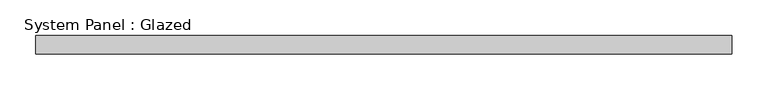
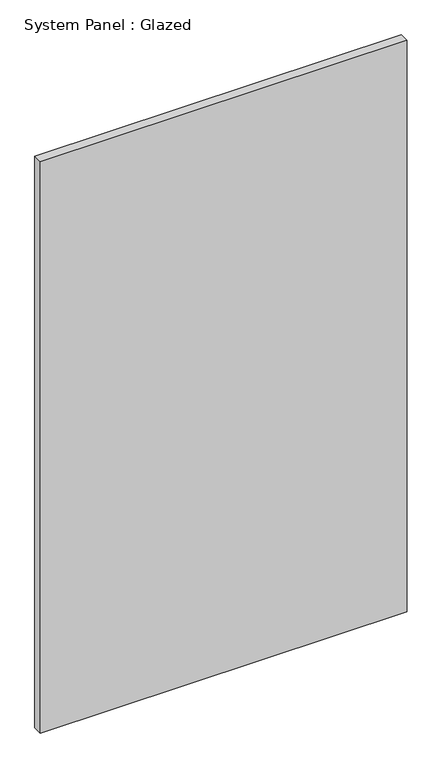
"""IFC4 building model written with IfcOpenShell, lengths in millimetres: plate geometry, System Panel : Glazed."""

from ifc_helpers import new_model, si_unit, origin, origin_with_axes, place, context, project, spatial, polyline, outline, extrude, source, transform, mapped, element, save


def system_panel_glazed_0e829309(model_context):
    return source(origin(), model_context, "Body", "SweptSolid", [
        extrude(outline(polyline([(485.775, 19.05), (-485.775, 19.05), (-485.775, 44.45), (485.775, 44.45), (485.775, 19.05)])), origin_with_axes(), (0.0, 0.0, 1.0), 1599.8137367),
    ])


if __name__ == "__main__":
    model = new_model("IFC4")
    model_context = context("Model", 3, world=origin())
    ifc_project = project(units=[si_unit("LENGTHUNIT", "METRE", prefix="MILLI")], contexts=[model_context])
    site = spatial("IfcSite", under=ifc_project)
    building = spatial("IfcBuilding", under=site)
    placement = place(None, origin())
    system_panel_glazed_shape = system_panel_glazed_0e829309(model_context)
    element("IfcPlate", 1, ObjectType="System Panel : Glazed", at=placement, inside=building, context=model_context, shape_type="MappedRepresentation", body=[
        mapped(system_panel_glazed_shape, transform((0.0, 0.0, 0.0), x_axis=(1.0, 0.0, 0.0), y_axis=(0.0, 1.0, 0.0), z_axis=(0.0, 0.0, 1.0))),
    ])
    save(model, "model.ifc")

# Revit data of these elements
# Type "System Panel : Glazed"
#   Construction Type Id = "GSP4R"
#   Analytic Construction = "1/8 in Pilkington single glazing"
#   Visual Light Transmittance = 0.9
#   Solar Heat Gain Coefficient = 0.86
#   Heat Transfer Coefficient (U) = 1.18115 BTU/(h·ft²·°F)
#   Define Thermal Properties by = 1
# Element 1 (IfcPlate, "System Panel : Glazed")
#   Materials on its faces: "Glass"
# Materials
#   "Glass": class "Glass", colour RGB 0 128 192, transparency 0.75, Description = "Soda Lime Glass", Cost = 0
